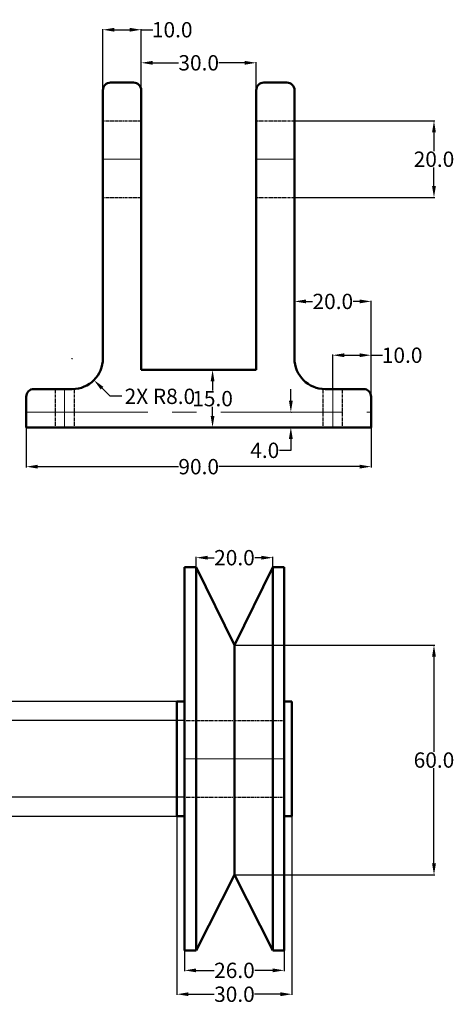
# Model space of a CAD drawing. Units: inches. Extents: x 639 to 969, y 329 to 654.
# Tile 2 of 2: x 856 to 969, y 395 to 652. Entities that reach past the tile are written whole.
import ezdxf

# ---------------------------------------------------------------- set-up
doc = ezdxf.new("R2010")
doc.units = ezdxf.units.IN
doc.header["$MEASUREMENT"] = 0
doc.linetypes.add('CENTER', pattern=[50.8, 31.75, -6.35, 6.35, -6.35])
doc.linetypes.add('HIDDEN', pattern=[0.375, 0.25, -0.125])
for name, color, linetype, lineweight in [('M-CNTR', 1, 'CENTER', 18), ('M-DIMS', 3, 'Continuous', 25), ('M-HIDN', 2, 'HIDDEN', 25), ('M-OUTL', 7, 'Continuous', 50)]:
    doc.layers.add(name, color=color, linetype=linetype, lineweight=lineweight)
doc.styles.get("Standard").update_dxf_attribs({"font": 'arial.ttf'})
doc.dimstyles.get("Standard").update_dxf_attribs({"dimtxt": 4, "dimasz": 3, "dimexe": 0.18, "dimexo": 0.0625, "dimgap": 0.09, "dimtad": 0, "dimtih": 1, "dimtoh": 1, "dimdec": 1, "dimzin": 0, "dimdsep": 46, "dimtxsty": 'Standard', "dimcen": 0.09, "dimadec": 0, "dimazin": 0, "dimtfac": 1, "dimtdec": 1, "dimtofl": 0, "dimtmove": 0, "dimatfit": 3, "dimfxl": 1, "dimtolj": 1, "dimtzin": 0, "dimarcsym": 0})

# ---------------------------------------------------------------- blocks, each defined once
blk = doc.blocks.new('*D1')
at = {"layer": 'Defpoints', "color": 0, "transparency": 16777216}
for p in [(887.41, 648.95), (877.41, 631.11), (887.41, 631.11)]:
    blk.add_point(p, dxfattribs=at)
at = {"layer": 'M-DIMS', "color": 0, "lineweight": -2, "transparency": 16777216}
for p, q in [((877.41, 631.18), (877.41, 649.13)), ((880.41, 648.95), (884.41, 648.95)), ((887.41, 631.18), (887.41, 649.13)), ((887.41, 648.95), (890.41, 648.95))]:
    blk.add_line(p, q, dxfattribs=at)
at = {"layer": 'M-DIMS', "color": 0, "transparency": 16777216}
for points in [[(880.41, 649.45), (880.41, 648.45), (877.41, 648.95)], [(884.41, 649.45), (884.41, 648.45), (887.41, 648.95)]]:
    blk.add_solid(points, dxfattribs=at)
at = {"layer": 'M-DIMS', "color": 0, "transparency": 16777216, "insert": (895.5, 648.95), "char_height": 4, "attachment_point": 5}
blk.add_mtext('\\A1;10.0', dxfattribs=at)
blk = doc.blocks.new('*D2')
at = {"layer": 'Defpoints', "color": 0, "transparency": 16777216}
for p in [(917.41, 640.32), (887.41, 627.46), (917.41, 627.46)]:
    blk.add_point(p, dxfattribs=at)
at = {"layer": 'M-DIMS', "color": 0, "lineweight": -2, "transparency": 16777216}
for p, q in [((887.41, 627.52), (887.41, 640.5)), ((890.41, 640.32), (897.14, 640.32)), ((914.41, 640.32), (907.69, 640.32)), ((917.41, 627.52), (917.41, 640.5))]:
    blk.add_line(p, q, dxfattribs=at)
at = {"layer": 'M-DIMS', "color": 0, "transparency": 16777216}
for points in [[(890.41, 640.82), (890.41, 639.82), (887.41, 640.32)], [(914.41, 640.82), (914.41, 639.82), (917.41, 640.32)]]:
    blk.add_solid(points, dxfattribs=at)
at = {"layer": 'M-DIMS', "color": 0, "transparency": 16777216, "insert": (902.41, 640.32), "char_height": 4, "attachment_point": 5}
blk.add_mtext('\\A1;30.0', dxfattribs=at)
blk = doc.blocks.new('*D3')
at = {"layer": 'Defpoints', "color": 0, "transparency": 16777216}
for p in [(947.41, 578.03), (927.41, 575.22), (947.41, 548.08)]:
    blk.add_point(p, dxfattribs=at)
at = {"layer": 'M-DIMS', "color": 0, "lineweight": -2, "transparency": 16777216}
for p, q in [((927.41, 575.28), (927.41, 578.21)), ((930.41, 578.03), (932.1, 578.03)), ((944.41, 578.03), (942.72, 578.03)), ((947.41, 548.15), (947.41, 578.21))]:
    blk.add_line(p, q, dxfattribs=at)
at = {"layer": 'M-DIMS', "color": 0, "transparency": 16777216}
for points in [[(930.41, 578.53), (930.41, 577.53), (927.41, 578.03)], [(944.41, 578.53), (944.41, 577.53), (947.41, 578.03)]]:
    blk.add_solid(points, dxfattribs=at)
at = {"layer": 'M-DIMS', "color": 0, "transparency": 16777216, "insert": (937.41, 578.03), "char_height": 4, "attachment_point": 5}
blk.add_mtext('\\A1;20.0', dxfattribs=at)
blk = doc.blocks.new('*D4')
at = {"layer": 'Defpoints', "color": 0, "transparency": 16777216}
for p in [(926.46, 549.16), (926.46, 545.16), (926.46, 545.16)]:
    blk.add_point(p, dxfattribs=at)
at = {"layer": 'M-DIMS', "color": 0, "lineweight": -2, "transparency": 16777216}
for p, q in [((926.46, 552.16), (926.46, 555.16)), ((926.52, 549.16), (926.64, 549.16)), ((926.52, 545.16), (926.64, 545.16)), ((926.46, 542.16), (926.46, 539.16)), ((926.46, 539.16), (923.46, 539.16))]:
    blk.add_line(p, q, dxfattribs=at)
at = {"layer": 'M-DIMS', "color": 0, "transparency": 16777216}
for points in [[(925.96, 552.16), (926.96, 552.16), (926.46, 549.16)], [(925.96, 542.16), (926.96, 542.16), (926.46, 545.16)]]:
    blk.add_solid(points, dxfattribs=at)
at = {"layer": 'M-DIMS', "color": 0, "transparency": 16777216, "insert": (919.65, 539.16), "char_height": 4, "attachment_point": 5}
blk.add_mtext('\\A1;4.0', dxfattribs=at)
blk = doc.blocks.new('*D5')
at = {"layer": 'Defpoints', "color": 0, "transparency": 16777216}
for p in [(947.41, 563.99), (937.41, 555.16), (947.41, 552.39)]:
    blk.add_point(p, dxfattribs=at)
at = {"layer": 'M-DIMS', "color": 0, "lineweight": -2, "transparency": 16777216}
for p, q in [((937.41, 555.22), (937.41, 564.17)), ((940.41, 563.99), (944.41, 563.99)), ((947.41, 552.45), (947.41, 564.17)), ((947.41, 563.99), (950.41, 563.99))]:
    blk.add_line(p, q, dxfattribs=at)
at = {"layer": 'M-DIMS', "color": 0, "transparency": 16777216}
for points in [[(940.41, 564.49), (940.41, 563.49), (937.41, 563.99)], [(944.41, 564.49), (944.41, 563.49), (947.41, 563.99)]]:
    blk.add_solid(points, dxfattribs=at)
at = {"layer": 'M-DIMS', "color": 0, "transparency": 16777216, "insert": (955.5, 563.99), "char_height": 4, "attachment_point": 5}
blk.add_mtext('\\A1;10.0', dxfattribs=at)
blk = doc.blocks.new('*D6')
at = {"layer": 'Defpoints', "color": 0, "transparency": 16777216}
for p in [(903.97, 560.16), (903.38, 545.16), (906.03, 545.16)]:
    blk.add_point(p, dxfattribs=at)
at = {"layer": 'M-DIMS', "color": 0, "lineweight": -2, "transparency": 16777216}
for p, q in [((904.03, 560.16), (906.21, 560.16)), ((906.03, 557.16), (906.03, 554.79)), ((906.03, 548.16), (906.03, 550.52)), ((903.44, 545.16), (906.21, 545.16))]:
    blk.add_line(p, q, dxfattribs=at)
at = {"layer": 'M-DIMS', "color": 0, "transparency": 16777216}
for points in [[(905.53, 557.16), (906.53, 557.16), (906.03, 560.16)], [(905.53, 548.16), (906.53, 548.16), (906.03, 545.16)]]:
    blk.add_solid(points, dxfattribs=at)
at = {"layer": 'M-DIMS', "color": 0, "transparency": 16777216, "insert": (906.03, 552.66), "char_height": 4, "attachment_point": 5}
blk.add_mtext('\\A1;15.0', dxfattribs=at)
blk = doc.blocks.new('*D7')
at = {"layer": 'Defpoints', "color": 0, "transparency": 16777216}
for p in [(857.41, 545.16), (947.41, 545.16), (947.41, 534.9)]:
    blk.add_point(p, dxfattribs=at)
at = {"layer": 'M-DIMS', "color": 0, "lineweight": -2, "transparency": 16777216}
for p, q in [((857.41, 545.09), (857.41, 534.72)), ((947.41, 545.09), (947.41, 534.72)), ((860.41, 534.9), (897.13, 534.9)), ((944.41, 534.9), (907.69, 534.9))]:
    blk.add_line(p, q, dxfattribs=at)
at = {"layer": 'M-DIMS', "color": 0, "transparency": 16777216}
for points in [[(860.41, 535.4), (860.41, 534.4), (857.41, 534.9)], [(944.41, 535.4), (944.41, 534.4), (947.41, 534.9)]]:
    blk.add_solid(points, dxfattribs=at)
at = {"layer": 'M-DIMS', "color": 0, "transparency": 16777216, "insert": (902.41, 534.9), "char_height": 4, "attachment_point": 5}
blk.add_mtext('\\A1;90.0', dxfattribs=at)
blk = doc.blocks.new('*D26')
at = {"layer": 'Defpoints', "color": 0, "transparency": 16777216}
for p in [(898.74, 408.62), (924.74, 408.62), (924.74, 403.41)]:
    blk.add_point(p, dxfattribs=at)
at = {"layer": 'M-DIMS', "color": 0, "lineweight": -2, "transparency": 16777216}
for p, q in [((898.74, 408.56), (898.74, 403.23)), ((924.74, 408.56), (924.74, 403.23)), ((901.74, 403.41), (906.42, 403.41)), ((921.74, 403.41), (917.05, 403.41))]:
    blk.add_line(p, q, dxfattribs=at)
at = {"layer": 'M-DIMS', "color": 0, "transparency": 16777216}
for points in [[(901.74, 403.91), (901.74, 402.91), (898.74, 403.41)], [(921.74, 403.91), (921.74, 402.91), (924.74, 403.41)]]:
    blk.add_solid(points, dxfattribs=at)
at = {"layer": 'M-DIMS', "color": 0, "transparency": 16777216, "insert": (911.74, 403.41), "char_height": 4, "attachment_point": 5}
blk.add_mtext('\\A1;26.0', dxfattribs=at)
blk = doc.blocks.new('*D27')
at = {"layer": 'Defpoints', "color": 0, "transparency": 16777216}
for p in [(896.74, 443.62), (926.74, 443.62), (926.74, 397.18)]:
    blk.add_point(p, dxfattribs=at)
at = {"layer": 'M-DIMS', "color": 0, "lineweight": -2, "transparency": 16777216}
for p, q in [((896.74, 443.56), (896.74, 397)), ((926.74, 443.56), (926.74, 397)), ((899.74, 397.18), (906.46, 397.18)), ((923.74, 397.18), (917.01, 397.18))]:
    blk.add_line(p, q, dxfattribs=at)
at = {"layer": 'M-DIMS', "color": 0, "transparency": 16777216}
for points in [[(899.74, 397.68), (899.74, 396.68), (896.74, 397.18)], [(923.74, 397.68), (923.74, 396.68), (926.74, 397.18)]]:
    blk.add_solid(points, dxfattribs=at)
at = {"layer": 'M-DIMS', "color": 0, "transparency": 16777216, "insert": (911.74, 397.18), "char_height": 4, "attachment_point": 5}
blk.add_mtext('\\A1;30.0', dxfattribs=at)
blk = doc.blocks.new('*D28')
at = {"layer": 'Defpoints', "color": 0, "transparency": 16777216}
for p in [(921.74, 511.14), (901.74, 508.62), (921.74, 508.62)]:
    blk.add_point(p, dxfattribs=at)
at = {"layer": 'M-DIMS', "color": 0, "lineweight": -2, "transparency": 16777216}
for p, q in [((901.74, 508.68), (901.74, 511.32)), ((904.74, 511.14), (906.42, 511.14)), ((918.74, 511.14), (917.05, 511.14)), ((921.74, 508.68), (921.74, 511.32))]:
    blk.add_line(p, q, dxfattribs=at)
at = {"layer": 'M-DIMS', "color": 0, "transparency": 16777216}
for points in [[(904.74, 511.64), (904.74, 510.64), (901.74, 511.14)], [(918.74, 511.64), (918.74, 510.64), (921.74, 511.14)]]:
    blk.add_solid(points, dxfattribs=at)
at = {"layer": 'M-DIMS', "color": 0, "transparency": 16777216, "insert": (911.74, 511.14), "char_height": 4, "attachment_point": 5}
blk.add_mtext('\\A1;20.0', dxfattribs=at)
blk = doc.blocks.new('*D32')
at = {"layer": 'Defpoints', "color": 0, "transparency": 16777216}
for p in [(927.41, 625.16), (963.81, 625.16), (927.41, 605.16)]:
    blk.add_point(p, dxfattribs=at)
at = {"layer": 'M-DIMS', "color": 0, "lineweight": -2, "transparency": 16777216}
for p, q in [((927.47, 625.16), (963.99, 625.16)), ((963.81, 622.16), (963.81, 617.29)), ((963.81, 608.16), (963.81, 613.02)), ((927.47, 605.16), (963.99, 605.16))]:
    blk.add_line(p, q, dxfattribs=at)
at = {"layer": 'M-DIMS', "color": 0, "transparency": 16777216}
for points in [[(963.31, 622.16), (964.31, 622.16), (963.81, 625.16)], [(963.31, 608.16), (964.31, 608.16), (963.81, 605.16)]]:
    blk.add_solid(points, dxfattribs=at)
at = {"layer": 'M-DIMS', "color": 0, "transparency": 16777216, "insert": (963.81, 615.16), "char_height": 4, "attachment_point": 5}
blk.add_mtext('\\A1;20.0', dxfattribs=at)
blk = doc.blocks.new('*D33')
at = {"layer": 'Defpoints', "color": 0, "transparency": 16777216}
for p in [(911.74, 488.31), (963.81, 488.31), (911.74, 428.31)]:
    blk.add_point(p, dxfattribs=at)
at = {"layer": 'M-DIMS', "color": 0, "lineweight": -2, "transparency": 16777216}
for p, q in [((911.8, 488.31), (963.99, 488.31)), ((963.81, 485.31), (963.81, 460.44)), ((963.81, 431.31), (963.81, 456.18)), ((911.8, 428.31), (963.99, 428.31))]:
    blk.add_line(p, q, dxfattribs=at)
at = {"layer": 'M-DIMS', "color": 0, "transparency": 16777216}
for points in [[(963.31, 485.31), (964.31, 485.31), (963.81, 488.31)], [(963.31, 431.31), (964.31, 431.31), (963.81, 428.31)]]:
    blk.add_solid(points, dxfattribs=at)
at = {"layer": 'M-DIMS', "color": 0, "transparency": 16777216, "insert": (963.81, 458.31), "char_height": 4, "attachment_point": 5}
blk.add_mtext('\\A1;60.0', dxfattribs=at)
blk = doc.blocks.new('*D34')
at = {"layer": 'Defpoints', "color": 0, "transparency": 16777216}
for p in [(659.03, 473.62), (896.74, 473.62), (896.74, 443.62)]:
    blk.add_point(p, dxfattribs=at)
at = {"layer": 'M-DIMS', "color": 0, "lineweight": -2, "transparency": 16777216}
for p, q in [((896.67, 473.62), (658.85, 473.62)), ((659.03, 470.62), (659.03, 460.75)), ((659.03, 446.62), (659.03, 456.49)), ((896.67, 443.62), (658.85, 443.62))]:
    blk.add_line(p, q, dxfattribs=at)
at = {"layer": 'M-DIMS', "color": 0, "transparency": 16777216}
for points in [[(658.53, 470.62), (659.53, 470.62), (659.03, 473.62)], [(658.53, 446.62), (659.53, 446.62), (659.03, 443.62)]]:
    blk.add_solid(points, dxfattribs=at)
at = {"layer": 'M-DIMS', "color": 0, "transparency": 16777216, "insert": (659.03, 458.62), "char_height": 4, "attachment_point": 5}
blk.add_mtext('\\A1;30.0', dxfattribs=at)
blk = doc.blocks.new('*D35')
at = {"layer": 'Defpoints', "color": 0, "transparency": 16777216}
for p in [(659.03, 468.62), (898.74, 468.62), (898.74, 448.62)]:
    blk.add_point(p, dxfattribs=at)
at = {"layer": 'M-DIMS', "color": 0, "lineweight": -2, "transparency": 16777216}
for p, q in [((898.67, 468.62), (658.85, 468.62)), ((659.03, 465.62), (659.03, 460.75)), ((659.03, 451.62), (659.03, 456.49)), ((898.67, 448.62), (658.85, 448.62))]:
    blk.add_line(p, q, dxfattribs=at)
at = {"layer": 'M-DIMS', "color": 0, "transparency": 16777216}
for points in [[(658.53, 465.62), (659.53, 465.62), (659.03, 468.62)], [(658.53, 451.62), (659.53, 451.62), (659.03, 448.62)]]:
    blk.add_solid(points, dxfattribs=at)
at = {"layer": 'M-DIMS', "color": 0, "transparency": 16777216, "insert": (659.03, 458.62), "char_height": 4, "attachment_point": 5}
blk.add_mtext('\\A1;20.0', dxfattribs=at)
blk = doc.blocks.new('*D37')
at = {"layer": 'Defpoints', "color": 0, "transparency": 16777216}
for p in [(869.41, 563.16), (875.07, 557.5)]:
    blk.add_point(p, dxfattribs=at)
at = {"layer": 'M-DIMS', "color": 0, "lineweight": -2, "transparency": 16777216}
for p, q in [((869.32, 563.16), (869.5, 563.16)), ((869.41, 563.07), (869.41, 563.25)), ((879.31, 553.26), (877.19, 555.38)), ((882.31, 553.26), (879.31, 553.26))]:
    blk.add_line(p, q, dxfattribs=at)
at = {"layer": 'M-DIMS', "color": 0, "transparency": 16777216}
blk.add_solid([(877.54, 555.73), (876.84, 555.03), (875.07, 557.5)], dxfattribs=at)
at = {"layer": 'M-DIMS', "color": 0, "transparency": 16777216, "insert": (892.28, 553.26), "char_height": 4, "attachment_point": 5}
blk.add_mtext('\\A1;2X R8.0', dxfattribs=at)

msp = doc.modelspace()

# ---------------------------------------------------------------- linework, layer by layer
at = {"layer": 'M-CNTR'}
for p, q in [((877.412, 615.157), (887.412, 615.157)), ((917.412, 615.157), (927.412, 615.157)), ((867.412, 555.157), (867.412, 545.157)), ((937.412, 545.157), (937.412, 555.157)), ((857.412, 549.157), (947.412, 549.157)), ((898.736, 458.621), (924.736, 458.621))]:
    msp.add_line(p, q, dxfattribs=at)
at = {"layer": 'M-HIDN'}
for p, q in [((877.412, 625.157), (887.412, 625.157)), ((917.412, 625.157), (927.412, 625.157)), ((877.412, 605.157), (887.412, 605.157)), ((917.412, 605.157), (927.412, 605.157)), ((864.912, 555.157), (864.912, 545.157)), ((869.912, 555.157), (869.912, 545.157)), ((934.912, 545.157), (934.912, 555.157)), ((939.912, 545.157), (939.912, 555.157)), ((898.736, 468.621), (924.736, 468.621)), ((898.736, 448.621), (924.736, 448.621))]:
    msp.add_line(p, q, dxfattribs=at)
at = {"layer": 'M-OUTL'}
for p, q in [((879.412, 635.157), (885.412, 635.157)), ((919.412, 635.157), (925.412, 635.157)), ((877.412, 633.157), (877.412, 563.157)), ((887.412, 633.157), (887.412, 560.157)), ((917.412, 560.157), (917.412, 633.157)), ((927.412, 563.157), (927.412, 633.157)), ((887.412, 560.157), (917.412, 560.157)), ((857.412, 553.157), (857.412, 545.157)), ((869.412, 555.157), (859.412, 555.157)), ((945.412, 555.157), (935.412, 555.157)), ((947.412, 545.157), (947.412, 553.157)), ((857.412, 545.157), (947.412, 545.157)), ((898.736, 508.621), (901.736, 508.621)), ((898.736, 508.621), (898.736, 408.621)), ((901.736, 508.621), (901.736, 408.621)), ((911.736, 488.312), (901.736, 508.621)), ((911.736, 488.312), (921.736, 508.621)), ((921.736, 508.621), (921.736, 408.621)), ((921.736, 508.621), (924.736, 508.621)), ((924.736, 508.621), (924.736, 408.621)), ((911.736, 488.312), (911.736, 428.312)), ((896.736, 473.621), (898.736, 473.621)), ((896.736, 473.621), (896.736, 443.621)), ((924.736, 473.621), (926.736, 473.621)), ((926.736, 473.621), (926.736, 443.621)), ((896.736, 443.621), (898.736, 443.621)), ((924.736, 443.621), (926.736, 443.621)), ((901.736, 408.621), (911.736, 428.312)), ((911.736, 428.312), (921.736, 408.621)), ((898.736, 408.621), (901.736, 408.621)), ((921.736, 408.621), (924.736, 408.621))]:
    msp.add_line(p, q, dxfattribs=at)
for centre, radius, start, end in [((879.412, 633.157), 2, 90, 180), ((885.412, 633.157), 2, 0, 90), ((919.412, 633.157), 2, 90, 180), ((925.412, 633.157), 2, 0, 90), ((869.412, 563.157), 8, 270, 0), ((935.412, 563.157), 8, 180, 270), ((859.412, 553.157), 2, 90, 180), ((945.412, 553.157), 2, 0, 90)]:
    msp.add_arc(centre, radius, start, end, dxfattribs=at)

# ---------------------------------------------------------------- dimensions: what is measured, and where the dimension line sits
at = {"layer": 'M-DIMS'}
for base, p1, p2, picture, middle in [((887.412, 648.952), (877.412, 631.113), (887.412, 631.113), '*D1', (895.502, 648.952)), ((917.412, 640.325), (887.412, 627.457), (917.412, 627.457), '*D2', (902.412, 640.325)), ((947.412, 578.028), (927.412, 575.221), (947.412, 548.084), '*D3', (937.412, 578.028)), ((947.412, 563.986), (937.412, 555.157), (947.412, 552.388), '*D5', (955.502, 563.986)), ((947.412, 534.9), (857.412, 545.157), (947.412, 545.157), '*D7', (902.412, 534.9)), ((921.736, 511.139), (901.736, 508.621), (921.736, 508.621), '*D28', (911.736, 511.139)), ((926.736, 397.176), (896.736, 443.621), (926.736, 443.621), '*D27', (911.736, 397.176)), ((924.736, 403.414), (898.736, 408.621), (924.736, 408.621), '*D26', (911.736, 403.414))]:
    dim = msp.add_linear_dim(base=base, p1=p1, p2=p2, dimstyle='Standard', override={"dimclrd": 0, "dimclre": 0, "dimclrt": 0}, dxfattribs=at)
    dim.commit()
    dim.dimension.update_dxf_attribs({"geometry": picture, "text_midpoint": middle})
for base, p1, p2, override, picture, middle in [((963.812, 625.157), (927.412, 605.157), (927.412, 625.157), {"dimdec": 1, "dimlfac": 1, "dimrnd": 0, "dimzin": 0, "dimdsep": 46, "dimlunit": 2}, '*D32', (963.812, 615.157)), ((906.027, 545.157), (903.969, 560.157), (903.381, 545.157), {"dimclrd": 0, "dimclre": 0, "dimclrt": 0}, '*D6', (906.027, 552.657)), ((926.459, 545.157), (926.459, 549.157), (926.459, 545.157), {"dimclrd": 0, "dimclre": 0, "dimclrt": 0}, '*D4', (919.654, 539.157)), ((963.812, 488.312), (911.736, 428.312), (911.736, 488.312), {"dimdec": 1, "dimlfac": 1, "dimrnd": 0, "dimzin": 0, "dimdsep": 46, "dimlunit": 2}, '*D33', (963.812, 458.312)), ((659.029, 473.621), (896.736, 443.621), (896.736, 473.621), {"dimdec": 1, "dimlfac": 1, "dimrnd": 0, "dimzin": 0, "dimdsep": 46, "dimlunit": 2}, '*D34', (659.029, 458.621)), ((659.029, 468.621), (898.736, 448.621), (898.736, 468.621), {"dimdec": 1, "dimlfac": 1, "dimrnd": 0, "dimzin": 0, "dimdsep": 46, "dimlunit": 2}, '*D35', (659.029, 458.621))]:
    dim = msp.add_linear_dim(base=base, p1=p1, p2=p2, angle=90, dimstyle='Standard', override=override, dxfattribs=at)
    dim.commit()
    dim.dimension.update_dxf_attribs({"geometry": picture, "text_midpoint": middle})
dim = msp.add_radius_dim(center=(869.412, 563.157), mpoint=(875.069, 557.5), text='2X <>', dimstyle='Standard', override={"dimdec": 1, "dimlfac": 1, "dimrnd": 0, "dimzin": 0, "dimdsep": 46, "dimlunit": 2}, dxfattribs=at)
dim.commit()
dim.dimension.update_dxf_attribs({"geometry": '*D37', "text_midpoint": (892.281, 553.257)})

doc.saveas('drawing.dxf')
